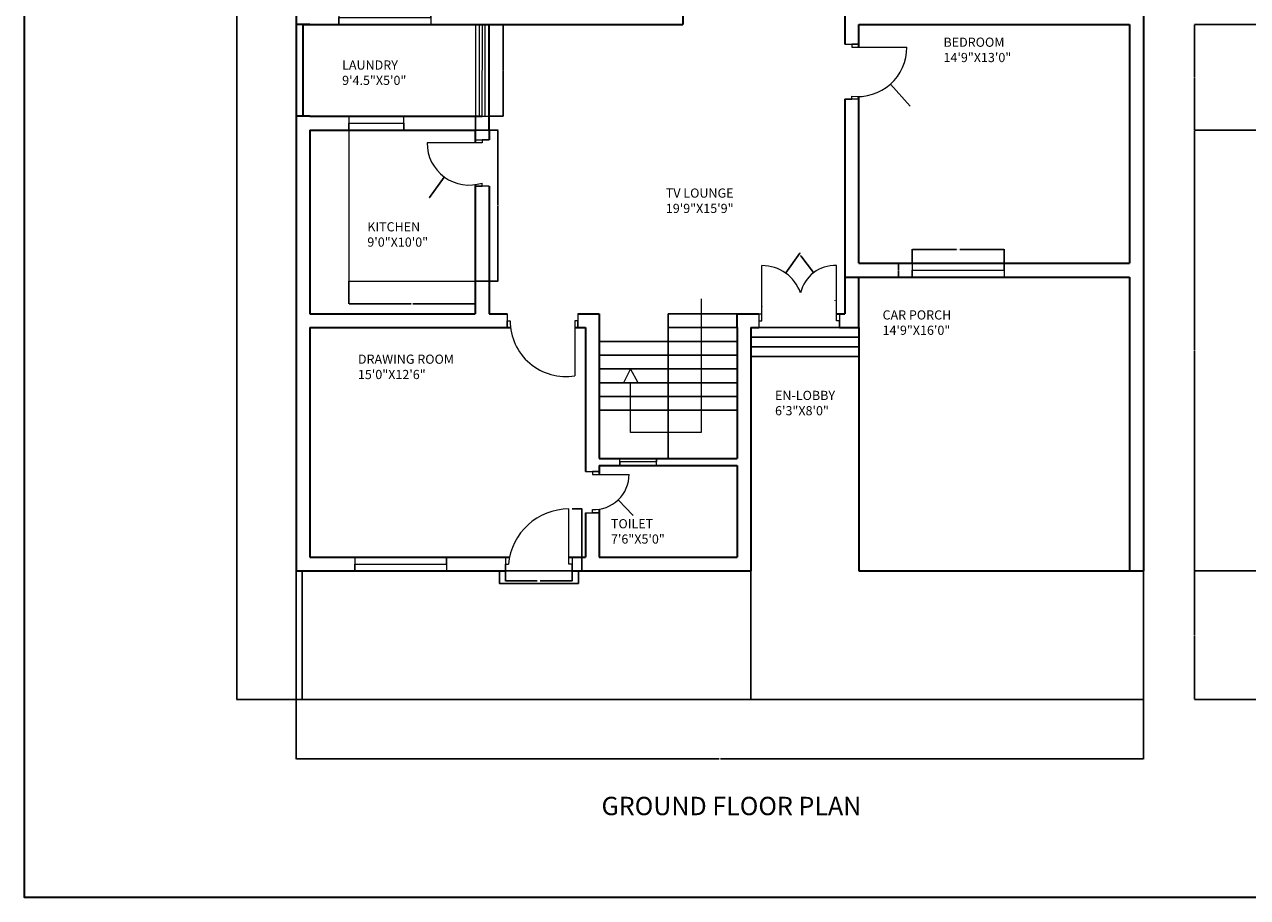
# Model space of a CAD drawing. Units: inches. Extents: x 2014 to 3678, y 870 to 2323.
# Tile 1 of 7: x 2014 to 2813, y 870 to 1440. Entities that reach past the tile are written whole.
import ezdxf

# ---------------------------------------------------------------- set-up
doc = ezdxf.new("R2010")
doc.units = ezdxf.units.IN
for name, color, linetype, lineweight in [('A-ANNO-DIMS', 2, 'Continuous', 18), ('A-ANNO-SYMB', 2, 'Continuous', 18), ('A-ANNO-TEXT', 7, 'Continuous', 18), ('A-ANNO-TTLB', 7, 'Continuous', 35), ('A-AREA-IDEN', 7, 'Continuous', 18), ('A-DOOR', 3, 'Continuous', 18), ('A-FLOR-FIXT', 8, 'Continuous', 18), ('A-FLOR-STRS', 7, 'Continuous', 25), ('A-GLAZ', 4, 'Continuous', 18), ('A-SITE', 8, 'Continuous', 25), ('A-WALL', 7, 'Continuous', 35)]:
    doc.layers.add(name, color=color, linetype=linetype, lineweight=lineweight)
doc.styles.get("Standard").update_dxf_attribs({"font": 'arial.ttf'})
doc.dimstyles.get("Standard").update_dxf_attribs({"dimtxt": 0.18, "dimasz": 0.18, "dimexe": 0.18, "dimexo": 0.0625, "dimgap": 0.09, "dimtad": 0, "dimtih": 1, "dimtoh": 1, "dimdec": 4, "dimzin": 0, "dimdsep": 46, "dimtxsty": 'Standard', "dimcen": 0.09, "dimadec": 0, "dimazin": 0, "dimtfac": 1, "dimtdec": 4, "dimtofl": 0, "dimtmove": 0, "dimatfit": 3, "dimfxl": 1, "dimtolj": 1, "dimtzin": 0, "dimarcsym": 0})

# ---------------------------------------------------------------- blocks, each defined once
blk = doc.blocks.new('DOOR-BED-SE-36')
for p, q in [((0, 36.03), (9, 36.03)), ((9, 36.03), (4.5, 36.03)), ((4.5, 36.03), (4.5, 34.03)), ((4.5, 34.03), (40.5, 34.03)), ((9, 0), (0, 0)), ((0, 0), (4.5, 0)), ((4.5, 0), (4.5, 2))]:
    blk.add_line(p, q)
blk.add_arc((8.25, 34.03), 32.25, 263.31406, 0)
blk = doc.blocks.new('DOOR-DRAWING-36')
for p, q in [((0, 40.98), (0, 31.98)), ((46.34, 40.98), (46.34, 31.98)), ((0, 31.98), (0, 36.48)), ((0, 36.48), (2, 36.48)), ((46.34, 36.48), (44.34, 36.48)), ((44.34, 36.48), (44.34, 0.48)), ((46.34, 31.98), (46.34, 36.48))]:
    blk.add_line(p, q)
blk.add_arc((38.48, 36.48), 36.48, 180, 279.25798)
blk = doc.blocks.new('DOOR-BATH-FRONT-24')
for p, q in [((0, 27), (9, 27)), ((9, 27), (4.5, 27)), ((4.5, 27), (4.5, 25)), ((4.5, 25), (28.5, 25)), ((4.5, 0), (4.5, 2)), ((0, 0), (9, 0)), ((9, 0), (4.5, 0))]:
    blk.add_line(p, q)
blk.add_arc((5.48, 25), 23.02, 267.56902, 0)
blk = doc.blocks.new('DOOR-FRONT-36')
for p, q in [((41.48, 4.5), (41.48, 40.5)), ((0, 9), (0, 0)), ((43.48, 9), (43.48, 0)), ((0, 0), (0, 4.5)), ((0, 4.5), (2, 4.5)), ((43.48, 4.5), (41.48, 4.5)), ((43.48, 0), (43.48, 4.5))]:
    blk.add_line(p, q)
blk.add_arc((41.48, 0.85), 39.65, 90, 174.72305)
blk = doc.blocks.new('DOOR-KITCHEN-36')
for p, q in [((12, 28.21), (0, 28.21)), ((36, 28.21), (12, 28.21)), ((31.5, 30.21), (40.5, 30.21)), ((40.5, 30.21), (36, 30.21)), ((36, 30.21), (36, 28.21)), ((36, 0), (36, 2)), ((40.5, 0), (31.5, 0)), ((31.5, 0), (36, 0))]:
    blk.add_line(p, q)
blk.add_arc((27.54, 28.21), 27.54, 180, 287.89435)
blk = doc.blocks.new('WIN-60')
for p, q in [((0, 9), (0, 0)), ((60, 4.5), (60, 9)), ((60, 9), (60, 0)), ((0, 0), (0, 4.5)), ((0, 4.5), (60, 4.5))]:
    blk.add_line(p, q)
blk = doc.blocks.new('VENT-24')
for p, q in [((0, 24), (4.5, 24)), ((4.5, 24), (2.25, 24)), ((2.25, 24), (2.25, 0)), ((2.25, 0), (0, 0)), ((0, 0), (4.5, 0))]:
    blk.add_line(p, q)
blk = doc.blocks.new('WIN-36')
for p, q in [((0, 9), (0, 0)), ((36, 0), (36, 9)), ((0, 0), (0, 4.5)), ((0, 4.5), (36, 4.5)), ((36, 4.5), (36, 0))]:
    blk.add_line(p, q)
blk = doc.blocks.new('GLAZ-LAUNDRY')
for p, q in [((9, 60), (0, 60)), ((0, 60), (0, 0)), ((4.5, 60), (2.5, 60)), ((2.5, 60), (2.5, 0)), ((4.35, 0), (4.5, 60)), ((6.35, 0), (6.35, 60)), ((8, 60), (7, 60)), ((9, 60), (8, 60)), ((0, 0), (4.35, 0)), ((2.5, 0), (4.35, 0)), ((4.35, 0), (9, 0.03)), ((7.27, 0.02), (9, 0.03)), ((4.35, 0), (6.35, 0))]:
    blk.add_line(p, q)
blk = doc.blocks.new('STAIR-HALF-TURN')
for p, q in [((45, 0), (45, 94.5)), ((45, 94.5), (90, 94.5)), ((45, 85.5), (90, 85.5)), ((45, 76.5), (0, 76.5)), ((45, 76.5), (90, 76.5)), ((45, 67.5), (0, 67.5)), ((45, 67.5), (90, 67.5)), ((45, 58.5), (0, 58.5)), ((45, 58.5), (90, 58.5)), ((45, 49.5), (0, 49.5)), ((45, 49.5), (90, 49.5)), ((45, 40.5), (0, 40.5)), ((45, 40.5), (90, 40.5)), ((45, 31.5), (0, 31.5)), ((45, 31.5), (90, 31.5)), ((90, 0), (0, 0))]:
    blk.add_line(p, q)
blk = doc.blocks.new('STAIR-DIRECTION')
for p, q in [((50.73, 87.32), (50.73, 0)), ((4.61, 41.51), (0, 32.51)), ((9.52, 32.51), (4.61, 41.51)), ((0, 32.51), (9.52, 32.51)), ((4.61, 0), (4.61, 32.51)), ((50.73, 0), (4.61, 0))]:
    blk.add_line(p, q)
blk = doc.blocks.new('STEPS-LOBBY')
for points in [[(0, 18.9), (70.5, 18.9), (70.5, 12.6), (0, 12.6)], [(0, 12.6), (70.5, 12.6), (70.5, 6.3), (0, 6.3)], [(0, 6.3), (70.5, 6.3), (70.5, 0), (0, 0)]]:
    blk.add_lwpolyline(points, close=True)
blk = doc.blocks.new('COUNTER-KITCHEN-L')
for p, q in [((0, 98.61), (0, 0)), ((0, 0), (82.65, 0))]:
    blk.add_line(p, q)
blk = doc.blocks.new('DOOR-LOBBY-PAIR')
for p, q in [((2, 4.5), (2, 40.5)), ((50.71, 4.5), (50.71, 40.5)), ((0, 9), (0, 0)), ((0, 9), (2, 9)), ((52.71, 9), (52.71, 0)), ((0, 4.5), (2, 4.5)), ((52.71, 4.5), (50.71, 4.5)), ((52.71, 0), (52.71, 4.5))]:
    blk.add_line(p, q)
for centre, radius, start, end in [((2, 13.8), 26.7, 19.35098, 90), ((49.6, 17.54), 22.98, 87.23183, 167.17299)]:
    blk.add_arc(centre, radius, start, end)
blk = doc.blocks.new('*D30')
at = {"layer": 'A-ANNO-DIMS', "color": 0, "lineweight": -2, "transparency": 16777216}
for p, q in [((2594, 1284.23), (2594, 1293.35)), ((2594.18, 1293.17), (2622.89, 1293.17)), ((2653.82, 1293.17), (2625.12, 1293.17)), ((2654, 1284.23), (2654, 1293.35))]:
    blk.add_line(p, q, dxfattribs=at)
at = {"layer": 'A-ANNO-DIMS', "color": 0, "transparency": 16777216}
for points in [[(2594.18, 1293.2), (2594.18, 1293.14), (2594, 1293.17)], [(2653.82, 1293.2), (2653.82, 1293.14), (2654, 1293.17)]]:
    blk.add_solid(points, dxfattribs=at)
at = {"layer": 'Defpoints', "color": 0, "transparency": 16777216}
for p in [(2654, 1293.17), (2594, 1284.17), (2654, 1284.17)]:
    blk.add_point(p, dxfattribs=at)
at = {"layer": 'A-ANNO-DIMS', "color": 0, "transparency": 16777216, "insert": (2624, 1293.17), "char_height": 0.18, "attachment_point": 5}
blk.add_mtext('\\A1;WINDOW 60 TYP.', dxfattribs=at)
blk = doc.blocks.new('*D31')
at = {"layer": 'A-ANNO-DIMS', "color": 0, "lineweight": -2, "transparency": 16777216}
for p, q in [((2593.94, 1284.17), (2584.82, 1284.17)), ((2585, 1283.99), (2585, 1279.85)), ((2585, 1275.35), (2585, 1279.48)), ((2593.94, 1275.17), (2584.82, 1275.17))]:
    blk.add_line(p, q, dxfattribs=at)
at = {"layer": 'A-ANNO-DIMS', "color": 0, "transparency": 16777216}
for points in [[(2584.97, 1283.99), (2585.03, 1283.99), (2585, 1284.17)], [(2584.97, 1275.35), (2585.03, 1275.35), (2585, 1275.17)]]:
    blk.add_solid(points, dxfattribs=at)
at = {"layer": 'Defpoints', "color": 0, "transparency": 16777216}
for p in [(2585, 1284.17), (2594, 1284.17), (2594, 1275.17)]:
    blk.add_point(p, dxfattribs=at)
at = {"layer": 'A-ANNO-DIMS', "color": 0, "transparency": 16777216, "insert": (2585, 1279.67), "char_height": 0.18, "attachment_point": 5}
blk.add_mtext('\\A1;9 TYP.', dxfattribs=at)
blk = doc.blocks.new('*D50')
at = {"layer": 'A-ANNO-DIMS', "color": 0, "lineweight": -2, "transparency": 16777216}
for p, q in [((2328.3, 1083.1), (2328.3, 1076.46)), ((2371.77, 1083.1), (2371.77, 1076.46)), ((2328.48, 1076.64), (2349.1, 1076.64)), ((2371.59, 1076.64), (2350.97, 1076.64))]:
    blk.add_line(p, q, dxfattribs=at)
at = {"layer": 'A-ANNO-DIMS', "color": 0, "transparency": 16777216}
for points in [[(2328.48, 1076.67), (2328.48, 1076.61), (2328.3, 1076.64)], [(2371.59, 1076.67), (2371.59, 1076.61), (2371.77, 1076.64)]]:
    blk.add_solid(points, dxfattribs=at)
at = {"layer": 'Defpoints', "color": 0, "transparency": 16777216}
for p in [(2328.3, 1083.17), (2371.77, 1083.17), (2371.77, 1076.64)]:
    blk.add_point(p, dxfattribs=at)
at = {"layer": 'A-ANNO-DIMS', "color": 0, "transparency": 16777216, "insert": (2350.03, 1076.64), "char_height": 0.18, "attachment_point": 5}
blk.add_mtext('\\A1;DOOR 43 TYP.', dxfattribs=at)
blk = doc.blocks.new('*D51')
at = {"layer": 'A-ANNO-DIMS', "color": 0, "lineweight": -2, "transparency": 16777216}
for p, q in [((2371.84, 1123.67), (2378.47, 1123.67)), ((2378.29, 1123.49), (2378.29, 1103.6)), ((2378.29, 1083.35), (2378.29, 1103.24)), ((2371.84, 1083.17), (2378.47, 1083.17))]:
    blk.add_line(p, q, dxfattribs=at)
at = {"layer": 'A-ANNO-DIMS', "color": 0, "transparency": 16777216}
for points in [[(2378.26, 1123.49), (2378.32, 1123.49), (2378.29, 1123.67)], [(2378.26, 1083.35), (2378.32, 1083.35), (2378.29, 1083.17)]]:
    blk.add_solid(points, dxfattribs=at)
at = {"layer": 'Defpoints', "color": 0, "transparency": 16777216}
for p in [(2371.77, 1123.67), (2378.29, 1123.67), (2371.77, 1083.17)]:
    blk.add_point(p, dxfattribs=at)
at = {"layer": 'A-ANNO-DIMS', "color": 0, "transparency": 16777216, "insert": (2378.29, 1103.42), "char_height": 0.18, "attachment_point": 5}
blk.add_mtext('\\A1;41 TYP.', dxfattribs=at)
blk = doc.blocks.new('*D62')
at = {"layer": 'A-ANNO-DIMS', "color": 0, "lineweight": -2, "transparency": 16777216}
for p, q in [((2317.78, 1440.17), (2326.89, 1440.17)), ((2326.71, 1439.99), (2326.71, 1410.35)), ((2326.71, 1380.34), (2326.71, 1409.98)), ((2317.78, 1380.16), (2326.89, 1380.16))]:
    blk.add_line(p, q, dxfattribs=at)
at = {"layer": 'A-ANNO-DIMS', "color": 0, "transparency": 16777216}
for points in [[(2326.68, 1439.99), (2326.74, 1439.99), (2326.71, 1440.17)], [(2326.68, 1380.34), (2326.74, 1380.34), (2326.71, 1380.16)]]:
    blk.add_solid(points, dxfattribs=at)
at = {"layer": 'Defpoints', "color": 0, "transparency": 16777216}
for p in [(2317.71, 1440.17), (2326.71, 1440.17), (2317.71, 1380.16)]:
    blk.add_point(p, dxfattribs=at)
at = {"layer": 'A-ANNO-DIMS', "color": 0, "transparency": 16777216, "insert": (2326.71, 1410.16), "char_height": 0.18, "attachment_point": 5}
blk.add_mtext('\\A1;GLAZING 60 TYP.', dxfattribs=at)
blk = doc.blocks.new('*D63')
at = {"layer": 'A-ANNO-DIMS', "color": 0, "lineweight": -2, "transparency": 16777216}
for p, q in [((2308.71, 1380.1), (2308.71, 1370.98)), ((2317.71, 1380.1), (2317.71, 1370.98)), ((2308.89, 1371.16), (2312.76, 1371.16)), ((2317.53, 1371.16), (2313.67, 1371.16))]:
    blk.add_line(p, q, dxfattribs=at)
at = {"layer": 'A-ANNO-DIMS', "color": 0, "transparency": 16777216}
for points in [[(2308.89, 1371.19), (2308.89, 1371.13), (2308.71, 1371.16)], [(2317.53, 1371.19), (2317.53, 1371.13), (2317.71, 1371.16)]]:
    blk.add_solid(points, dxfattribs=at)
at = {"layer": 'Defpoints', "color": 0, "transparency": 16777216}
for p in [(2308.71, 1380.16), (2317.71, 1380.16), (2317.71, 1371.16)]:
    blk.add_point(p, dxfattribs=at)
at = {"layer": 'A-ANNO-DIMS', "color": 0, "transparency": 16777216, "insert": (2313.21, 1371.16), "char_height": 0.18, "attachment_point": 5}
blk.add_mtext('\\A1;9 TYP.', dxfattribs=at)
blk = doc.blocks.new('*D68')
at = {"layer": 'A-ANNO-DIMS', "color": 0, "lineweight": -2, "transparency": 16777216}
for p, q in [((2308.62, 1371.17), (2323.53, 1371.17)), ((2323.35, 1370.99), (2323.35, 1322.04)), ((2323.35, 1272.74), (2323.35, 1321.68)), ((2308.62, 1272.56), (2323.53, 1272.56))]:
    blk.add_line(p, q, dxfattribs=at)
at = {"layer": 'A-ANNO-DIMS', "color": 0, "transparency": 16777216}
for points in [[(2323.32, 1370.99), (2323.38, 1370.99), (2323.35, 1371.17)], [(2323.32, 1272.74), (2323.38, 1272.74), (2323.35, 1272.56)]]:
    blk.add_solid(points, dxfattribs=at)
at = {"layer": 'Defpoints', "color": 0, "transparency": 16777216}
for p in [(2308.56, 1371.17), (2323.35, 1371.17), (2308.56, 1272.56)]:
    blk.add_point(p, dxfattribs=at)
at = {"layer": 'A-ANNO-DIMS', "color": 0, "transparency": 16777216, "insert": (2323.35, 1321.86), "char_height": 0.18, "attachment_point": 5}
blk.add_mtext('\\A1;COUNTER 99 TYP.', dxfattribs=at)
blk = doc.blocks.new('*D69')
at = {"layer": 'A-ANNO-DIMS', "color": 0, "lineweight": -2, "transparency": 16777216}
for p, q in [((2225.91, 1272.49), (2225.91, 1257.58)), ((2308.56, 1272.49), (2308.56, 1257.58)), ((2226.09, 1257.76), (2266.71, 1257.76)), ((2308.38, 1257.76), (2267.77, 1257.76))]:
    blk.add_line(p, q, dxfattribs=at)
at = {"layer": 'A-ANNO-DIMS', "color": 0, "transparency": 16777216}
for points in [[(2226.09, 1257.79), (2226.09, 1257.73), (2225.91, 1257.76)], [(2308.38, 1257.79), (2308.38, 1257.73), (2308.56, 1257.76)]]:
    blk.add_solid(points, dxfattribs=at)
at = {"layer": 'Defpoints', "color": 0, "transparency": 16777216}
for p in [(2225.91, 1272.56), (2308.56, 1272.56), (2308.56, 1257.76)]:
    blk.add_point(p, dxfattribs=at)
at = {"layer": 'A-ANNO-DIMS', "color": 0, "transparency": 16777216, "insert": (2267.24, 1257.76), "char_height": 0.18, "attachment_point": 5}
blk.add_mtext('\\A1;83 TYP.', dxfattribs=at)
blk = doc.blocks.new('*D86')
at = {"layer": 'A-ANNO-DIMS', "color": 0, "lineweight": -2, "transparency": 16777216}
for p, q in [((2191.56, 999.1), (2191.56, 960.29)), ((2745.06, 999.1), (2745.06, 960.29)), ((2191.74, 960.47), (2467.92, 960.47)), ((2744.88, 960.47), (2468.71, 960.47))]:
    blk.add_line(p, q, dxfattribs=at)
at = {"layer": 'A-ANNO-DIMS', "color": 0, "transparency": 16777216}
for points in [[(2191.74, 960.5), (2191.74, 960.44), (2191.56, 960.47)], [(2744.88, 960.5), (2744.88, 960.44), (2745.06, 960.47)]]:
    blk.add_solid(points, dxfattribs=at)
at = {"layer": 'Defpoints', "color": 0, "transparency": 16777216}
for p in [(2191.56, 999.17), (2745.06, 999.17), (2745.06, 960.47)]:
    blk.add_point(p, dxfattribs=at)
at = {"layer": 'A-ANNO-DIMS', "color": 0, "transparency": 16777216, "insert": (2468.31, 960.47), "char_height": 0.18, "attachment_point": 5}
blk.add_mtext('\\A1;553.5', dxfattribs=at)
blk = doc.blocks.new('*D87')
at = {"layer": 'A-ANNO-DIMS', "color": 0, "lineweight": -2, "transparency": 16777216}
for p, q in [((2191.5, 1683.17), (2152.68, 1683.17)), ((2152.86, 1682.99), (2152.86, 1341.35)), ((2152.86, 999.35), (2152.86, 1340.98)), ((2191.5, 999.17), (2152.68, 999.17))]:
    blk.add_line(p, q, dxfattribs=at)
at = {"layer": 'A-ANNO-DIMS', "color": 0, "transparency": 16777216}
for points in [[(2152.83, 1682.99), (2152.89, 1682.99), (2152.86, 1683.17)], [(2152.83, 999.35), (2152.89, 999.35), (2152.86, 999.17)]]:
    blk.add_solid(points, dxfattribs=at)
at = {"layer": 'Defpoints', "color": 0, "transparency": 16777216}
for p in [(2152.86, 1683.17), (2191.56, 1683.17), (2191.56, 999.17)]:
    blk.add_point(p, dxfattribs=at)
at = {"layer": 'A-ANNO-DIMS', "color": 0, "transparency": 16777216, "insert": (2152.86, 1341.17), "char_height": 0.18, "attachment_point": 5}
blk.add_mtext('\\A1;684', dxfattribs=at)
blk = doc.blocks.new('*D93')
at = {"layer": 'A-ANNO-DIMS', "color": 0, "lineweight": -2, "transparency": 16777216}
for p, q in [((2848.61, 1083.17), (2778.34, 1083.17)), ((2778.52, 1082.99), (2778.52, 1041.35)), ((2778.52, 999.35), (2778.52, 1040.98)), ((2848.61, 999.17), (2778.34, 999.17))]:
    blk.add_line(p, q, dxfattribs=at)
at = {"layer": 'A-ANNO-DIMS', "color": 0, "transparency": 16777216}
for points in [[(2778.49, 1082.99), (2778.55, 1082.99), (2778.52, 1083.17)], [(2778.49, 999.35), (2778.55, 999.35), (2778.52, 999.17)]]:
    blk.add_solid(points, dxfattribs=at)
at = {"layer": 'Defpoints', "color": 0, "transparency": 16777216}
for p in [(2778.52, 1083.17), (2848.67, 1083.17), (2848.67, 999.17)]:
    blk.add_point(p, dxfattribs=at)
at = {"layer": 'A-ANNO-DIMS', "color": 0, "transparency": 16777216, "insert": (2778.52, 1041.17), "char_height": 0.18, "attachment_point": 5}
blk.add_mtext('\\A1;84', dxfattribs=at)
blk = doc.blocks.new('*D94')
at = {"layer": 'A-ANNO-DIMS', "color": 0, "lineweight": -2, "transparency": 16777216}
for p, q in [((2857.61, 1371.17), (2778.34, 1371.17)), ((2778.52, 1370.99), (2778.52, 1227.35)), ((2778.52, 1083.35), (2778.52, 1226.98)), ((2848.61, 1083.17), (2778.34, 1083.17))]:
    blk.add_line(p, q, dxfattribs=at)
at = {"layer": 'A-ANNO-DIMS', "color": 0, "transparency": 16777216}
for points in [[(2778.49, 1370.99), (2778.55, 1370.99), (2778.52, 1371.17)], [(2778.49, 1083.35), (2778.55, 1083.35), (2778.52, 1083.17)]]:
    blk.add_solid(points, dxfattribs=at)
at = {"layer": 'Defpoints', "color": 0, "transparency": 16777216}
for p in [(2778.52, 1371.17), (2857.67, 1371.17), (2848.67, 1083.17)]:
    blk.add_point(p, dxfattribs=at)
at = {"layer": 'A-ANNO-DIMS', "color": 0, "transparency": 16777216, "insert": (2778.52, 1227.17), "char_height": 0.18, "attachment_point": 5}
blk.add_mtext('\\A1;288', dxfattribs=at)
blk = doc.blocks.new('*D95')
at = {"layer": 'A-ANNO-DIMS', "color": 0, "lineweight": -2, "transparency": 16777216}
for p, q in [((2848.61, 1440.17), (2778.34, 1440.17)), ((2778.52, 1439.99), (2778.52, 1405.85)), ((2778.52, 1371.35), (2778.52, 1405.48)), ((2857.61, 1371.17), (2778.34, 1371.17))]:
    blk.add_line(p, q, dxfattribs=at)
at = {"layer": 'A-ANNO-DIMS', "color": 0, "transparency": 16777216}
for points in [[(2778.49, 1439.99), (2778.55, 1439.99), (2778.52, 1440.17)], [(2778.49, 1371.35), (2778.55, 1371.35), (2778.52, 1371.17)]]:
    blk.add_solid(points, dxfattribs=at)
at = {"layer": 'Defpoints', "color": 0, "transparency": 16777216}
for p in [(2778.52, 1440.17), (2848.67, 1440.17), (2857.67, 1371.17)]:
    blk.add_point(p, dxfattribs=at)
at = {"layer": 'A-ANNO-DIMS', "color": 0, "transparency": 16777216, "insert": (2778.52, 1405.67), "char_height": 0.18, "attachment_point": 5}
blk.add_mtext('\\A1;69', dxfattribs=at)
blk = doc.blocks.new('*D125')
at = {"layer": 'A-ANNO-DIMS', "color": 0, "lineweight": -2, "transparency": 16777216}
for p, q in [((2558.22, 1425.31), (2558.4, 1425.31)), ((2558.31, 1425.22), (2558.31, 1425.4)), ((2592.61, 1386.76), (2579.87, 1401.08)), ((2592.79, 1386.76), (2592.61, 1386.76))]:
    blk.add_line(p, q, dxfattribs=at)
at = {"layer": 'A-ANNO-DIMS', "color": 0, "transparency": 16777216}
blk.add_solid([(2579.89, 1401.1), (2579.85, 1401.06), (2579.75, 1401.22)], dxfattribs=at)
at = {"layer": 'Defpoints', "color": 0, "transparency": 16777216}
for p in [(2558.31, 1425.31), (2579.75, 1401.22)]:
    blk.add_point(p, dxfattribs=at)
at = {"layer": 'A-ANNO-DIMS', "color": 0, "transparency": 16777216, "insert": (2593.34, 1386.76), "char_height": 0.18, "attachment_point": 5}
blk.add_mtext('\\A1;R32.246', dxfattribs=at)
blk = doc.blocks.new('*D126')
at = {"layer": 'A-ANNO-DIMS', "color": 0, "lineweight": -2, "transparency": 16777216}
for p, q in [((2304.51, 1362.76), (2304.69, 1362.76)), ((2304.6, 1362.67), (2304.6, 1362.85)), ((2278.67, 1327.14), (2288.29, 1340.35)), ((2278.49, 1327.14), (2278.67, 1327.14))]:
    blk.add_line(p, q, dxfattribs=at)
at = {"layer": 'A-ANNO-DIMS', "color": 0, "transparency": 16777216}
blk.add_solid([(2288.26, 1340.37), (2288.31, 1340.34), (2288.39, 1340.5)], dxfattribs=at)
at = {"layer": 'Defpoints', "color": 0, "transparency": 16777216}
for p in [(2304.6, 1362.76), (2288.39, 1340.5)]:
    blk.add_point(p, dxfattribs=at)
at = {"layer": 'A-ANNO-DIMS', "color": 0, "transparency": 16777216, "insert": (2278.01, 1327.14), "char_height": 0.18, "attachment_point": 5}
blk.add_mtext('\\A1;R27.54', dxfattribs=at)
blk = doc.blocks.new('*D127')
at = {"layer": 'A-ANNO-DIMS', "color": 0, "lineweight": -2, "transparency": 16777216}
for p, q in [((2520.58, 1290.82), (2511.42, 1277.9)), ((2520.76, 1290.82), (2520.58, 1290.82)), ((2495.78, 1255.96), (2495.96, 1255.96)), ((2495.87, 1255.87), (2495.87, 1256.05))]:
    blk.add_line(p, q, dxfattribs=at)
at = {"layer": 'A-ANNO-DIMS', "color": 0, "transparency": 16777216}
blk.add_solid([(2511.39, 1277.91), (2511.44, 1277.88), (2511.31, 1277.75)], dxfattribs=at)
at = {"layer": 'Defpoints', "color": 0, "transparency": 16777216}
for p in [(2511.31, 1277.75), (2495.87, 1255.96)]:
    blk.add_point(p, dxfattribs=at)
at = {"layer": 'A-ANNO-DIMS', "color": 0, "transparency": 16777216, "insert": (2521.17, 1290.82), "char_height": 0.18, "attachment_point": 5}
blk.add_mtext('\\A1;R26.7', dxfattribs=at)
blk = doc.blocks.new('*D129')
at = {"layer": 'A-ANNO-DIMS', "color": 0, "lineweight": -2, "transparency": 16777216}
for p, q in [((2385.95, 1146.26), (2386.13, 1146.26)), ((2386.04, 1146.17), (2386.04, 1146.35)), ((2411.53, 1119.66), (2402.09, 1129.5)), ((2411.71, 1119.66), (2411.53, 1119.66))]:
    blk.add_line(p, q, dxfattribs=at)
at = {"layer": 'A-ANNO-DIMS', "color": 0, "transparency": 16777216}
blk.add_solid([(2402.11, 1129.53), (2402.07, 1129.48), (2401.97, 1129.63)], dxfattribs=at)
at = {"layer": 'Defpoints', "color": 0, "transparency": 16777216}
for p in [(2386.04, 1146.26), (2401.97, 1129.63)]:
    blk.add_point(p, dxfattribs=at)
at = {"layer": 'A-ANNO-DIMS', "color": 0, "transparency": 16777216, "insert": (2412.26, 1119.66), "char_height": 0.18, "attachment_point": 5}
blk.add_mtext('\\A1;R23.023', dxfattribs=at)
blk = doc.blocks.new('*D130')
at = {"layer": 'A-ANNO-DIMS', "color": 0, "lineweight": -2, "transparency": 16777216}
for p, q in [((2521.06, 1289), (2521.24, 1289)), ((2521.24, 1289), (2529.47, 1278.16)), ((2543.39, 1259.71), (2543.57, 1259.71)), ((2543.48, 1259.62), (2543.48, 1259.8))]:
    blk.add_line(p, q, dxfattribs=at)
at = {"layer": 'A-ANNO-DIMS', "color": 0, "transparency": 16777216}
blk.add_solid([(2529.5, 1278.18), (2529.45, 1278.14), (2529.58, 1278.02)], dxfattribs=at)
at = {"layer": 'Defpoints', "color": 0, "transparency": 16777216}
for p in [(2529.58, 1278.02), (2543.48, 1259.71)]:
    blk.add_point(p, dxfattribs=at)
at = {"layer": 'A-ANNO-DIMS', "color": 0, "transparency": 16777216, "insert": (2520.51, 1289), "char_height": 0.18, "attachment_point": 5}
blk.add_mtext('\\A1;R22.983', dxfattribs=at)

msp = doc.modelspace()

# ---------------------------------------------------------------- linework, layer by layer
at = {"layer": 'A-ANNO-TTLB'}
msp.add_lwpolyline([(2014.0556, 2323.3638), (3678.0069, 2323.3638), (3678.0069, 869.855), (2014.0556, 869.855)], close=True, dxfattribs=at)
at = {"layer": 'A-FLOR-STRS'}
msp.add_lwpolyline([(2324.3435, 1083.1655), (2375.9267, 1083.1655), (2375.9267, 1075.091), (2324.3435, 1075.091)], close=True, dxfattribs=at)
at = {"layer": 'A-SITE'}
for p, q in [((2191.5607, 999.1655), (2191.5607, 1083.1655)), ((2195.5607, 999.1655), (2195.5607, 1083.1655)), ((2488.5607, 1083.1655), (2488.5607, 999.1655)), ((2745.0607, 1083.1655), (2745.0607, 999.1655)), ((2745.0607, 999.1655), (2191.5607, 999.1655)), ((2191.5607, 999.1655), (2193.5607, 999.1655)), ((2193.5607, 999.1655), (2195.5607, 999.1655))]:
    msp.add_line(p, q, dxfattribs=at)
at = {"layer": 'A-WALL'}
for p, q in [((2191.5607, 1683.1655), (2191.5607, 1083.1655)), ((2745.0607, 1683.1655), (2745.0607, 1083.1655)), ((2444.2554, 1449.1655), (2444.2554, 1440.1655)), ((2550.0607, 1453.8082), (2550.0607, 1440.1655)), ((2200.5607, 1440.1655), (2191.5607, 1440.1655)), ((2196.0607, 1380.1655), (2196.0607, 1440.1655)), ((2196.0607, 1440.1655), (2200.5607, 1440.1655)), ((2200.5607, 1440.1655), (2313.0607, 1440.1655)), ((2313.0607, 1440.1655), (2322.1008, 1440.1655)), ((2317.5607, 1371.1655), (2317.7142, 1440.1655)), ((2322.1008, 1440.1655), (2444.2554, 1440.1655)), ((2550.0607, 1440.1655), (2550.0607, 1427.3075)), ((2559.0607, 1440.1655), (2736.0607, 1440.1655)), ((2559.0607, 1425.3075), (2559.0607, 1440.1655)), ((2736.0607, 1440.1655), (2736.0607, 1284.1655)), ((2550.0607, 1391.2811), (2550.0607, 1275.1655)), ((2559.0607, 1284.1655), (2559.0607, 1393.0704)), ((2196.0607, 1380.1655), (2191.5607, 1380.1655)), ((2200.5607, 1380.1655), (2196.0607, 1380.1655)), ((2200.5607, 1380.1655), (2313.0607, 1380.1655)), ((2200.5607, 1371.1655), (2308.5607, 1371.1655)), ((2200.5607, 1371.1655), (2308.5607, 1371.1655)), ((2200.5607, 1371.1655), (2200.5607, 1251.1655)), ((2308.5607, 1371.1655), (2308.5607, 1362.764)), ((2317.5607, 1371.1655), (2317.5607, 1364.764)), ((2308.5607, 1335.512), (2308.5607, 1251.1655)), ((2317.5607, 1334.5577), (2317.5607, 1251.1655)), ((2559.0607, 1284.1655), (2736.0607, 1284.1655)), ((2550.0607, 1275.1655), (2559.0607, 1275.1655)), ((2550.0607, 1275.1655), (2550.0607, 1251.1655)), ((2559.0607, 1275.1655), (2736.0607, 1275.1655)), ((2559.0607, 1242.1655), (2559.0607, 1275.1655)), ((2736.0607, 1275.1655), (2736.0607, 1083.1655)), ((2200.5607, 1251.1655), (2308.5607, 1251.1655)), ((2317.5607, 1251.1655), (2329.3029, 1251.1655)), ((2375.6461, 1251.1655), (2389.5607, 1251.1655)), ((2389.5607, 1251.1655), (2389.5607, 1242.1655)), ((2479.5607, 1242.1655), (2479.5607, 1251.1655)), ((2479.5607, 1251.1655), (2493.8749, 1251.1655)), ((2544.5867, 1251.1655), (2550.0607, 1251.1655)), ((2200.5607, 1242.1655), (2308.5607, 1242.1655)), ((2200.5607, 1242.1655), (2200.5607, 1092.1655)), ((2308.5607, 1242.1655), (2317.5607, 1242.1655)), ((2317.5607, 1242.1655), (2331.5815, 1242.1655)), ((2373.6461, 1242.1655), (2380.5607, 1242.1655)), ((2380.5607, 1242.1655), (2380.5607, 1148.2566)), ((2389.5607, 1242.1655), (2389.5607, 1156.6655)), ((2479.5607, 1242.1655), (2479.5607, 1156.6655)), ((2488.5607, 1242.1655), (2488.5607, 1083.1655)), ((2488.5607, 1242.1655), (2493.8749, 1242.1655)), ((2546.5867, 1242.1655), (2550.0607, 1242.1655)), ((2550.0607, 1242.1655), (2559.0607, 1242.1655)), ((2559.0607, 1242.1655), (2559.0607, 1083.1655)), ((2389.5607, 1156.6655), (2479.5607, 1156.6655)), ((2389.5607, 1152.1655), (2479.5607, 1152.1655)), ((2389.5607, 1152.1655), (2389.5607, 1146.2566)), ((2479.5607, 1152.1655), (2479.5607, 1092.1655)), ((2380.5607, 1121.2539), (2380.5607, 1092.1655)), ((2389.5607, 1123.5044), (2389.5607, 1092.1655)), ((2200.5607, 1092.1655), (2330.9729, 1092.1655)), ((2369.7733, 1092.1655), (2380.5607, 1092.1655)), ((2389.5607, 1092.1655), (2479.5607, 1092.1655)), ((2191.5607, 1083.1655), (2328.295, 1083.1655)), ((2371.7733, 1083.1655), (2389.5607, 1083.1655)), ((2389.5607, 1083.1655), (2488.5607, 1083.1655)), ((2559.0607, 1083.1655), (2745.0607, 1083.1655)), ((2736.0607, 1083.1655), (2745.0607, 1083.1655))]:
    msp.add_line(p, q, dxfattribs=at)

# ---------------------------------------------------------------- block references
at = {"layer": 'A-ANNO-SYMB'}
msp.add_blockref('STAIR-DIRECTION', (2405.417, 1173.658), dxfattribs=at)
at = {"layer": 'A-DOOR'}
for name, p in [('DOOR-BED-SE-36', (2550.061, 1391.281)), ('DOOR-KITCHEN-36', (2277.061, 1334.558)), ('DOOR-LOBBY-PAIR', (2493.875, 1242.165)), ('DOOR-DRAWING-36', (2329.303, 1210.19)), ('DOOR-BATH-FRONT-24', (2380.561, 1121.254)), ('DOOR-FRONT-36', (2328.295, 1083.165))]:
    msp.add_blockref(name, p, dxfattribs=at)
at = {"layer": 'A-FLOR-FIXT'}
msp.add_blockref('COUNTER-KITCHEN-L', (2225.914, 1272.556), dxfattribs=at)
at = {"layer": 'A-FLOR-STRS'}
for name, p in [('STAIR-HALF-TURN', (2389.561, 1156.665)), ('STEPS-LOBBY', (2488.561, 1223.263))]:
    msp.add_blockref(name, p, dxfattribs=at)
at = {"layer": 'A-GLAZ'}
for name, p in [('WIN-60', (2219.4692, 1440.165)), ('GLAZ-LAUNDRY', (2308.714, 1380.161)), ('WIN-36', (2225.914, 1371.165)), ('WIN-60', (2594.0051, 1275.165)), ('WIN-60', (2229.86, 1083.165))]:
    msp.add_blockref(name, p, dxfattribs=at)
at = {"layer": 'A-GLAZ', "extrusion": (0, 0, -1), "zscale": -1, "rotation": 90}
msp.add_blockref('VENT-24', (-2402.9199, 1152.1658), dxfattribs=at)

# ---------------------------------------------------------------- texts
at = {"layer": 'A-ANNO-TEXT', "insert": (2391.046, 935.6516), "char_height": 12, "attachment_point": 1}
msp.add_mtext_dynamic_manual_height_columns('GROUND FLOOR PLAN', width=376.391584, gutter_width=12.5, heights=[0], dxfattribs=at)
at = {"layer": 'A-AREA-IDEN', "char_height": 6, "attachment_point": 1}
for s, width, insert in [('BEDROOM\\P14\'9"X13\'0"', 153.794334, (2614.4677, 1431.5827)), ('LAUNDRY\\P9\'4.5"X5\'0"', 118.46619, (2221.5811, 1416.6566)), ('TV LOUNGE\\P19\'9"X15\'9"', 90.929341, (2433.0581, 1333.0175)), ('KITCHEN\\P9\'0"X10\'0"', 114.925771, (2238.0524, 1311.0069)), ('CAR PORCH\\P14\'9"X16\'0"', 133.713748, (2574.6487, 1253.4161)), ('DRAWING ROOM\\P15\'0"X12\'6"', 157.648218, (2231.9125, 1224.5174)), ('EN-LOBBY\\P6\'3"X8\'0"', 72.973006, (2504.4201, 1200.8581)), ('TOILET\\P7\'6"X5\'0"', 85.899096, (2397.2167, 1117.031))]:
    msp.add_mtext_dynamic_manual_height_columns(s, width=width, gutter_width=12.5, heights=[0], dxfattribs=dict(at, insert=insert))

# ---------------------------------------------------------------- dimensions: what is measured, and where the dimension line sits
at = {"layer": 'A-ANNO-DIMS'}
for base, p1, p2, picture, middle in [((2152.8607, 1683.1655), (2191.5607, 999.1655), (2191.5607, 1683.1655), '*D87', (2152.8607, 1341.1655)), ((2778.5231, 1440.1655), (2857.6718, 1371.1655), (2848.6718, 1440.1655), '*D95', (2778.5231, 1405.6655)), ((2778.5231, 1371.1655), (2848.6718, 1083.1655), (2857.6718, 1371.1655), '*D94', (2778.5231, 1227.1655)), ((2778.5231, 1083.1655), (2848.6718, 999.1655), (2848.6718, 1083.1655), '*D93', (2778.5231, 1041.1655))]:
    dim = msp.add_linear_dim(base=base, p1=p1, p2=p2, angle=90, dimstyle='Standard', override={"dimdec": 0, "dimlfac": 1, "dimrnd": 0, "dimzin": 0, "dimdsep": 46, "dimlunit": 2}, dxfattribs=at)
    dim.commit()
    dim.dimension.update_dxf_attribs({"geometry": picture, "text_midpoint": middle})
for base, p1, p2, text, picture, middle in [((2326.715, 1440.1655), (2317.7142, 1380.1607), (2317.7142, 1440.1655), 'GLAZING <> TYP.', '*D62', (2326.715, 1410.1631)), ((2323.3521, 1371.1655), (2308.5607, 1272.5559), (2308.5607, 1371.1655), 'COUNTER <> TYP.', '*D68', (2323.3521, 1321.8607)), ((2585.0046, 1284.1655), (2594.0046, 1275.1655), (2594.0046, 1284.1655), '<> TYP.', '*D31', (2585.0046, 1279.6655)), ((2378.2949887681, 1123.6654745472), (2371.7732535982, 1083.1654745472), (2371.7732535982, 1123.6654745472), '<> TYP.', '*D51', (2378.2949887681, 1103.4154745472))]:
    dim = msp.add_linear_dim(base=base, p1=p1, p2=p2, angle=90, text=text, dimstyle='Standard', override={"dimdec": 0, "dimlfac": 1, "dimrnd": 0, "dimzin": 0, "dimdsep": 46, "dimlunit": 2}, dxfattribs=at)
    dim.commit()
    dim.dimension.update_dxf_attribs({"geometry": picture, "text_midpoint": middle})
for center, mpoint, override, picture, middle in [((2558.315, 1425.3075), (2579.7481, 1401.2159), {"dimdec": 3, "dimlfac": 1, "dimrnd": 0, "dimzin": 0, "dimdsep": 46, "dimlunit": 2}, '*D125', (2593.3377, 1386.7609)), ((2304.5992, 1362.764), (2288.3919, 1340.4999), {"dimdec": 2, "dimlfac": 1, "dimrnd": 0, "dimzin": 0, "dimdsep": 46, "dimlunit": 2}, '*D126', (2278.0081, 1327.1414)), ((2495.8749, 1255.9644), (2511.3137, 1277.7495), {"dimdec": 1, "dimlfac": 1, "dimrnd": 0, "dimzin": 0, "dimdsep": 46, "dimlunit": 2}, '*D127', (2521.1668, 1290.8206)), ((2543.4768, 1259.7095), (2529.5807, 1278.0154), {"dimdec": 3, "dimlfac": 1, "dimrnd": 0, "dimzin": 0, "dimdsep": 46, "dimlunit": 2}, '*D130', (2520.5133, 1288.999)), ((2386.0373, 1146.2566), (2401.9682, 1129.6348), {"dimdec": 3, "dimlfac": 1, "dimrnd": 0, "dimzin": 0, "dimdsep": 46, "dimlunit": 2}, '*D129', (2412.2565, 1119.6617))]:
    dim = msp.add_radius_dim(center=center, mpoint=mpoint, dimstyle='Standard', override=override, dxfattribs=at)
    dim.commit()
    dim.dimension.update_dxf_attribs({"geometry": picture, "text_midpoint": middle, "dimtype": 164})
for base, p1, p2, text, picture, middle in [((2317.7142, 1371.16), (2308.7142, 1380.1607), (2317.7142, 1380.1607), '<> TYP.', '*D63', (2313.2142, 1371.16)), ((2654.0046, 1293.1655), (2594.0046, 1284.1655), (2654.0046, 1284.1655), 'WINDOW <> TYP.', '*D30', (2624.0046, 1293.1655)), ((2308.5607, 1257.7644), (2225.9135, 1272.5559), (2308.5607, 1272.5559), '<> TYP.', '*D69', (2267.2371, 1257.7644)), ((2371.7733, 1076.6437), (2328.295, 1083.1655), (2371.7733, 1083.1655), 'DOOR <> TYP.', '*D50', (2350.0341, 1076.6437))]:
    dim = msp.add_linear_dim(base=base, p1=p1, p2=p2, text=text, dimstyle='Standard', override={"dimdec": 0, "dimlfac": 1, "dimrnd": 0, "dimzin": 0, "dimdsep": 46, "dimlunit": 2}, dxfattribs=at)
    dim.commit()
    dim.dimension.update_dxf_attribs({"geometry": picture, "text_midpoint": middle})
dim = msp.add_linear_dim(base=(2745.0607, 960.4655), p1=(2191.5607, 999.1655), p2=(2745.0607, 999.1655), dimstyle='Standard', override={"dimdec": 1, "dimlfac": 1, "dimrnd": 0, "dimzin": 0, "dimdsep": 46, "dimlunit": 2}, dxfattribs=at)
dim.commit()
dim.dimension.update_dxf_attribs({"geometry": '*D86', "text_midpoint": (2468.3107, 960.4655)})

doc.saveas('drawing.dxf')
